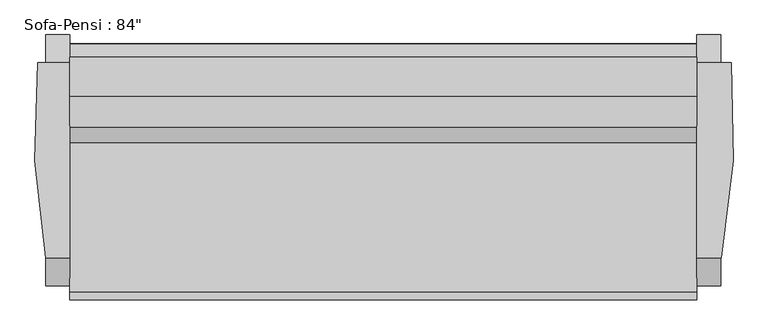
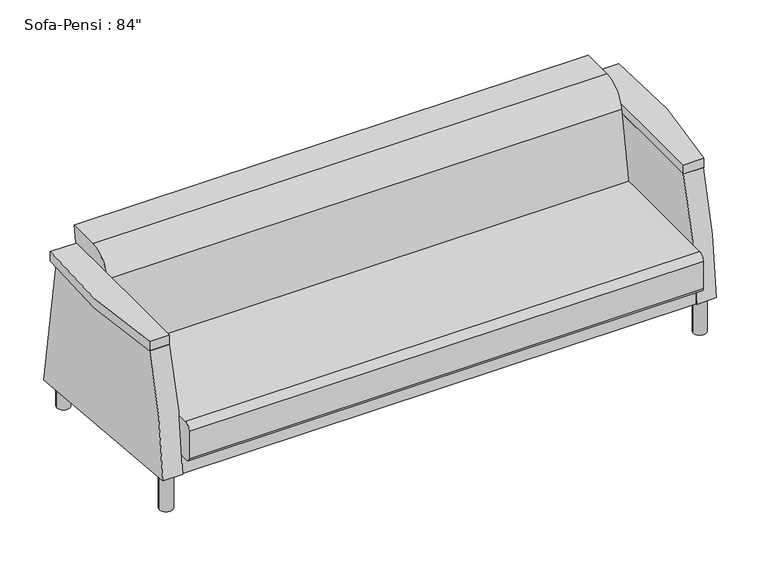
"""IFC4 building model written with IfcOpenShell, lengths in millimetres: furniture geometry."""

from ifc_helpers import new_model, si_unit, point, frame, frame_2d, origin, origin_with_axes, place, context, project, spatial, polyline, circle_curve, trimmed, segment, composite_curve, outline, extrude, source, transform, mapped, element, save


def furniture_4a9d42a7(model_context):
    return source(origin(), model_context, "Body", "SweptSolid", [
        extrude(outline(composite_curve([segment(trimmed(circle_curve(frame_2d((-116.5901639, 351.2509954)), 25.4), [point((-141.9901639, 351.2509954))], [point((-116.5901639, 376.6509954))], False, "CARTESIAN"), True, "CONTINUOUS"), segment(polyline([(-116.5901639, 376.6509954), (355.3895541, 376.6509954), (402.1988177, 642.1195211)]), True, "CONTINUOUS"), segment(trimmed(circle_curve(frame_2d((502.2552854, 624.4768662)), 101.6), [point((402.1988177, 642.1195211))], [point((502.2552854, 726.0768662))], False, "CARTESIAN"), True, "CONTINUOUS"), segment(polyline([(502.2552854, 726.0768662), (626.3344485, 726.0768662), (609.5377828, 620.1719187), (667.6541767, 224.2509954), (-126.1151639, 224.2509954)]), True, "CONTINUOUS"), segment(trimmed(circle_curve(frame_2d((-126.1151639, 240.1259954)), 15.875), [point((-126.1151639, 224.2509954))], [point((-141.9901639, 240.1259954))], False, "CARTESIAN"), True, "CONTINUOUS"), segment(polyline([(-141.9901639, 240.1259954), (-141.9901639, 351.2509954)]), True, "CONTINUOUS")], self_intersect=False)), frame((-711.99375, 0.0, 0.0), z_axis=(1.0, 0.0, 0.0), x_axis=(0.0, 1.0, 0.0)), (0.0, 0.0, 1.0), 1981.2),
        extrude(outline(composite_curve([segment(polyline([(696.2098361, 79.844579), (-97.7900405, 149.3105671)]), True, "CONTINUOUS"), segment(trimmed(circle_curve(frame_2d((1499.9783711, 99.5888442)), 1598.5418814), [point((-97.7900405, 149.3105671))], [point((-9.3943348, 626.0203985))], False, "CARTESIAN"), True, "CONTINUOUS"), segment(polyline([(-9.3943348, 626.0203985), (608.6917937, 626.0203985), (696.2098361, 79.844579)]), True, "CONTINUOUS")], self_intersect=False)), frame((1269.20625, 0.0, 0.0), z_axis=(1.0, 0.0, 0.0), x_axis=(0.0, 1.0, 0.0)), (0.0, 0.0, 1.0), 76.2),
        extrude(outline(composite_curve([segment(polyline([(-9.3943348, 626.0203985), (608.6917937, 626.0203985), (696.2098361, 79.844579), (-97.7900405, 149.3105671)]), True, "CONTINUOUS"), segment(trimmed(circle_curve(frame_2d((1499.9783711, 99.5888442)), 1598.5418814), [point((-97.7900405, 149.3105671))], [point((-9.3943348, 626.0203985))], False, "CARTESIAN"), True, "CONTINUOUS")], self_intersect=False)), frame((-788.19375, 0.0, 0.0), z_axis=(1.0, 0.0, 0.0), x_axis=(0.0, 1.0, 0.0)), (0.0, 0.0, 1.0), 76.2),
        extrude(outline(polyline([(1269.20625, 668.3047863), (1269.20625, -93.6952137), (-711.99375, -93.6952137), (-711.99375, 668.3047863), (1269.20625, 668.3047863)])), frame((0.0, 0.0, 148.0509954), z_axis=(0.0, 0.0, 1.0), x_axis=(1.0, 0.0, 0.0)), (0.0, 0.0, 1.0), 76.2),
        extrude(outline(composite_curve([segment(trimmed(circle_curve(frame_2d((-750.09375, -53.0901639)), 25.4), [point((-775.49375, -53.0901639))], [point((-724.69375, -53.0901639))], False, "CARTESIAN"), True, "CONTINUOUS"), segment(trimmed(circle_curve(frame_2d((-750.09375, -53.0901639)), 25.4), [point((-724.69375, -53.0901639))], [point((-775.49375, -53.0901639))], False, "CARTESIAN"), True, "CONTINUOUS")], self_intersect=False)), origin_with_axes(), (0.0, 0.0, 1.0), 148.43125),
        extrude(outline(composite_curve([segment(trimmed(circle_curve(frame_2d((-750.09375, 632.7098361)), 25.4), [point((-775.49375, 632.7098361))], [point((-724.69375, 632.7098361))], False, "CARTESIAN"), True, "CONTINUOUS"), segment(trimmed(circle_curve(frame_2d((-750.09375, 632.7098361)), 25.4), [point((-724.69375, 632.7098361))], [point((-775.49375, 632.7098361))], False, "CARTESIAN"), True, "CONTINUOUS")], self_intersect=False)), origin_with_axes(), (0.0, 0.0, 1.0), 148.43125),
        extrude(outline(composite_curve([segment(trimmed(circle_curve(frame_2d((1307.30625, 632.7098361)), 25.4), [point((1281.90625, 632.7098361))], [point((1332.70625, 632.7098361))], False, "CARTESIAN"), True, "CONTINUOUS"), segment(trimmed(circle_curve(frame_2d((1307.30625, 632.7098361)), 25.4), [point((1332.70625, 632.7098361))], [point((1281.90625, 632.7098361))], False, "CARTESIAN"), True, "CONTINUOUS")], self_intersect=False)), origin_with_axes(), (0.0, 0.0, 1.0), 148.43125),
        extrude(outline(composite_curve([segment(trimmed(circle_curve(frame_2d((1307.30625, -53.0901639)), 25.4), [point((1281.90625, -53.0901639))], [point((1332.70625, -53.0901639))], False, "CARTESIAN"), True, "CONTINUOUS"), segment(trimmed(circle_curve(frame_2d((1307.30625, -53.0901639)), 25.4), [point((1332.70625, -53.0901639))], [point((1281.90625, -53.0901639))], False, "CARTESIAN"), True, "CONTINUOUS")], self_intersect=False)), origin_with_axes(), (0.0, 0.0, 1.0), 148.43125),
        extrude(outline(composite_curve([segment(polyline([(-711.99375, -9.3943348), (-788.19375, -9.3943348)]), True, "CONTINUOUS"), segment(trimmed(circle_curve(frame_2d((1379.5527561, 389.2532985)), 2204.0972869), [point((-788.19375, -9.3943348))], [point((-813.59375, 608.6917935))], False, "CARTESIAN"), True, "CONTINUOUS"), segment(polyline([(-813.59375, 608.6917935), (-711.99375, 608.6917935), (-711.99375, -9.3943348)]), True, "CONTINUOUS")], self_intersect=False)), frame((0.0, 0.0, 626.0203985), z_axis=(0.0, 0.0, 1.0), x_axis=(1.0, 0.0, 0.0)), (0.0, 0.0, 1.0), 38.1),
        extrude(outline(composite_curve([segment(polyline([(1269.20625, -9.3943348), (1269.20625, 608.9395268), (1377.8864453, 608.9395268)]), True, "CONTINUOUS"), segment(trimmed(circle_curve(frame_2d((-821.3771494, 407.0073811)), 2208.514648), [point((1377.8864453, 608.9395268))], [point((1347.5273117, -9.3943348))], False, "CARTESIAN"), True, "CONTINUOUS"), segment(polyline([(1347.5273117, -9.3943348), (1269.20625, -9.3943348)]), True, "CONTINUOUS")], self_intersect=False)), frame((0.0, 0.0, 626.0203985), z_axis=(0.0, 0.0, 1.0), x_axis=(1.0, 0.0, 0.0)), (0.0, 0.0, 1.0), 38.1),
    ])


if __name__ == "__main__":
    model = new_model("IFC4")
    model_context = context("Model", 3, world=origin())
    ifc_project = project(units=[si_unit("LENGTHUNIT", "METRE", prefix="MILLI")], contexts=[model_context])
    site = spatial("IfcSite", under=ifc_project)
    building = spatial("IfcBuilding", under=site)
    placement = place(None, origin())
    furniture_shape = furniture_4a9d42a7(model_context)
    element("IfcFurniture", 1, ObjectType="Sofa-Pensi : 84\"", at=placement, inside=building, context=model_context, shape_type="MappedRepresentation", body=[
        mapped(furniture_shape, transform((0.0, 0.0, 0.0), x_axis=(1.0, 0.0, 0.0), y_axis=(0.0, 1.0, 0.0), z_axis=(0.0, 0.0, 1.0))),
    ])
    save(model, "model.ifc")

# Revit data of these elements
# Type "Sofa-Pensi : 84\""
#   Assembly Code = "E2020200"
#   Length = 7 ft
#   Frame Material = Cherry
#   Seat Material = Linen, Beige
#   Feet Material = Steel, Chrome Plated
#   Default Elevation = 0
# Element 1 (IfcFurniture, "Sofa-Pensi : 84\"")
#   Materials on its faces: "Cherry", "Linen, Beige", "Steel, Chrome Plated"
# Materials
#   "Cherry": class "Wood", colour RGB 226 177 128, transparency 0, Description = "Prunus Serotina", Cost = 0
#   "Linen, Beige": class "Textile", colour RGB 249 239 230, transparency 0, Description = "Linen, beige", Cost = 0
#   "Steel, Chrome Plated": class "Metal", colour RGB 17 17 17, transparency 0, Description = "Chromiuim plated steel", Cost = 0
